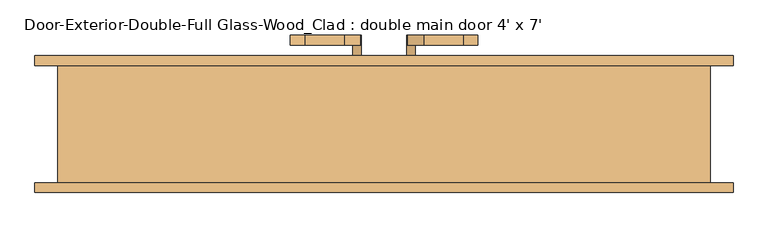
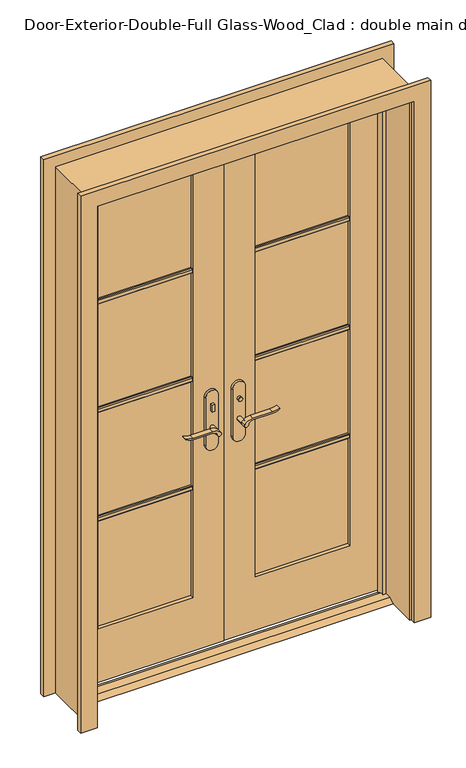
"""IFC4 building model written with IfcOpenShell, lengths in millimetres: door geometry, Door-Exterior-Double-Full Glass-Wood_Clad : double main door 4' x 7'."""

from ifc_helpers import new_model, si_unit, point, frame, frame_2d, origin, place, context, project, spatial, polyline, circle_curve, trimmed, segment, composite_curve, outline, extrude, faceted_brep, source, transform, mapped, element, save


def door_exterior_double_full_glass_wood_clad_double_main_door_4_3788f36b(model_context):
    return source(origin(), model_context, "Body", "SolidModel", [
        extrude(outline(polyline([(19.05, 12.7), (53.975, 12.7), (79.375, 0.0), (-6.35, 0.0), (19.05, 12.7)])), frame((-609.6, 0.0, 0.0), z_axis=(1.0, 0.0, 0.0), x_axis=(0.0, 1.0, 0.0)), (0.0, 0.0, 1.0), 1219.2),
        extrude(outline(polyline([(-47.4019111, 56.2), (-57.4019111, 56.2), (-57.4019111, 66.2), (-47.4019111, 66.2), (-47.4019111, 56.2)])), frame((0.0, 0.0, 981.9), z_axis=(0.0, 0.0, 1.0), x_axis=(1.0, 0.0, 0.0)), (0.0, 0.0, 1.0), 30.0),
        extrude(outline(composite_curve([segment(trimmed(circle_curve(frame_2d((996.9, -52.4019111)), 8.0), [point((996.9, -60.4019111))], [point((996.9, -44.4019111))], False, "CARTESIAN"), True, "CONTINUOUS"), segment(trimmed(circle_curve(frame_2d((996.9, -52.4019111)), 8.0), [point((996.9, -44.4019111))], [point((996.9, -60.4019111))], False, "CARTESIAN"), True, "CONTINUOUS")], self_intersect=False)), frame((0.0, 121.125, 0.0), z_axis=(0.0, 1.0, 0.0), x_axis=(0.0, 0.0, 1.0)), (0.0, 0.0, 1.0), 10.0),
        extrude(outline(composite_curve([segment(trimmed(circle_curve(frame_2d((897.1555521, -76.0694241)), 37.2832219), [point((919.0523287, -45.8937749))], [point((934.4, -77.7693445))], False, "CARTESIAN"), True, "CONTINUOUS"), segment(polyline([(934.4, -77.7693445), (934.4, -154.045502)]), True, "CONTINUOUS"), segment(trimmed(circle_curve(frame_2d((1017.6850638, -153.9791202)), 83.2850902), [point((934.4, -154.045502))], [point((939.4, -182.4019111))], True, "CARTESIAN"), True, "CONTINUOUS"), segment(polyline([(939.4, -182.4019111), (936.6135558, -182.4019111)]), True, "CONTINUOUS"), segment(trimmed(circle_curve(frame_2d((986.6709207, -150.4622499)), 59.3791355), [point((936.6135558, -182.4019111))], [point((927.4, -154.045502))], False, "CARTESIAN"), True, "CONTINUOUS"), segment(polyline([(927.4, -154.045502), (927.4, -77.7881013)]), True, "CONTINUOUS"), segment(trimmed(circle_curve(frame_2d((909.2738613, -77.7881013)), 18.1261387), [point((927.4, -77.7881013))], [point((914.4, -60.4019111))], True, "CARTESIAN"), True, "CONTINUOUS"), segment(trimmed(circle_curve(frame_2d((914.4, -52.4019111)), 8.0), [point((914.4, -60.4019111))], [point((919.0523287, -45.8937749))], False, "CARTESIAN"), True, "CONTINUOUS")], self_intersect=False)), frame((0.0, 16.2, 0.0), z_axis=(0.0, 1.0, 0.0), x_axis=(0.0, 0.0, 1.0)), (0.0, 0.0, 1.0), 20.0),
        extrude(outline(composite_curve([segment(trimmed(circle_curve(frame_2d((914.4, -52.4019111)), 8.0), [point((914.3999903, -60.4019111))], [point((919.0523287, -45.8937749))], False, "CARTESIAN"), True, "CONTINUOUS"), segment(trimmed(circle_curve(frame_2d((897.1555521, -76.0694241)), 37.2832219), [point((919.0523287, -45.8937749))], [point((934.4, -77.7693445))], False, "CARTESIAN"), True, "CONTINUOUS"), segment(polyline([(934.4, -77.7693445), (934.4, -154.045502)]), True, "CONTINUOUS"), segment(trimmed(circle_curve(frame_2d((1017.6850638, -153.9791202)), 83.2850902), [point((934.4, -154.045502))], [point((939.4, -182.4019111))], True, "CARTESIAN"), True, "CONTINUOUS"), segment(polyline([(939.4, -182.4019111), (936.6135558, -182.4019111)]), True, "CONTINUOUS"), segment(trimmed(circle_curve(frame_2d((986.6709207, -150.4622499)), 59.3791355), [point((936.6135558, -182.4019111))], [point((927.4, -154.045502))], False, "CARTESIAN"), True, "CONTINUOUS"), segment(polyline([(927.4, -154.045502), (927.4, -77.788099)]), True, "CONTINUOUS"), segment(trimmed(circle_curve(frame_2d((909.2738682, -77.788099)), 18.1261318), [point((927.4, -77.788099))], [point((914.3999903, -60.4019111))], True, "CARTESIAN"), True, "CONTINUOUS")], self_intersect=False)), frame((0.0, 151.125, 0.0), z_axis=(0.0, 1.0, 0.0), x_axis=(0.0, 0.0, 1.0)), (0.0, 0.0, 1.0), 20.0),
        extrude(outline(composite_curve([segment(trimmed(circle_curve(frame_2d((914.4, -52.4019111)), 8.0), [point((914.4, -60.4019111))], [point((914.4, -44.4019111))], False, "CARTESIAN"), True, "CONTINUOUS"), segment(trimmed(circle_curve(frame_2d((914.4, -52.4019111)), 8.0), [point((914.4, -44.4019111))], [point((914.4, -60.4019111))], False, "CARTESIAN"), True, "CONTINUOUS")], self_intersect=False)), frame((0.0, 36.2, 0.0), z_axis=(0.0, 1.0, 0.0), x_axis=(0.0, 0.0, 1.0)), (0.0, 0.0, 1.0), 30.0),
        extrude(outline(composite_curve([segment(trimmed(circle_curve(frame_2d((914.4, -52.4019111)), 8.0), [point((914.4, -60.4019111))], [point((914.4, -44.4019111))], False, "CARTESIAN"), True, "CONTINUOUS"), segment(trimmed(circle_curve(frame_2d((914.4, -52.4019111)), 8.0), [point((914.4, -44.4019111))], [point((914.4, -60.4019111))], False, "CARTESIAN"), True, "CONTINUOUS")], self_intersect=False)), frame((0.0, 121.125, 0.0), z_axis=(0.0, 1.0, 0.0), x_axis=(0.0, 0.0, 1.0)), (0.0, 0.0, 1.0), 30.0),
        extrude(outline(composite_curve([segment(polyline([(844.4, -27.4019111), (1039.4, -27.4019111)]), True, "CONTINUOUS"), segment(trimmed(circle_curve(frame_2d((1039.4, -52.4019111)), 25.0), [point((1039.4, -27.4019111))], [point((1039.4, -77.4019111))], False, "CARTESIAN"), True, "CONTINUOUS"), segment(polyline([(1039.4, -77.4019111), (844.4, -77.4019111)]), True, "CONTINUOUS"), segment(trimmed(circle_curve(frame_2d((844.4, -52.4019111)), 25.0), [point((844.4, -77.4019111))], [point((844.4, -27.4019111))], False, "CARTESIAN"), True, "CONTINUOUS")], self_intersect=False)), frame((0.0, 66.2, 0.0), z_axis=(0.0, 1.0, 0.0), x_axis=(0.0, 0.0, 1.0)), (0.0, 0.0, 1.0), 10.0),
        extrude(outline(composite_curve([segment(polyline([(844.4, -27.4019111), (1039.4, -27.4019111)]), True, "CONTINUOUS"), segment(trimmed(circle_curve(frame_2d((1039.4, -52.4019111)), 25.0), [point((1039.4, -27.4019111))], [point((1039.4, -77.4019111))], False, "CARTESIAN"), True, "CONTINUOUS"), segment(polyline([(1039.4, -77.4019111), (844.4, -77.4019111)]), True, "CONTINUOUS"), segment(trimmed(circle_curve(frame_2d((844.4, -52.4019111)), 25.0), [point((844.4, -77.4019111))], [point((844.4, -27.4019111))], False, "CARTESIAN"), True, "CONTINUOUS")], self_intersect=False)), frame((0.0, 111.125, 0.0), z_axis=(0.0, 1.0, 0.0), x_axis=(0.0, 0.0, 1.0)), (0.0, 0.0, 1.0), 10.0),
        extrude(outline(polyline([(47.3875, 131.125), (57.3875, 131.125), (57.3875, 121.125), (47.3875, 121.125), (47.3875, 131.125)])), frame((0.0, 0.0, 981.9), z_axis=(0.0, 0.0, 1.0), x_axis=(1.0, 0.0, 0.0)), (0.0, 0.0, 1.0), 30.0),
        extrude(outline(composite_curve([segment(trimmed(circle_curve(frame_2d((996.9, 52.3875)), 8.0), [point((996.9, 60.3875))], [point((996.9, 44.3875))], False, "CARTESIAN"), True, "CONTINUOUS"), segment(trimmed(circle_curve(frame_2d((996.9, 52.3875)), 8.0), [point((996.9, 44.3875))], [point((996.9, 60.3875))], False, "CARTESIAN"), True, "CONTINUOUS")], self_intersect=False)), frame((0.0, 56.2, 0.0), z_axis=(0.0, 1.0, 0.0), x_axis=(0.0, 0.0, 1.0)), (0.0, 0.0, 1.0), 10.0),
        extrude(outline(composite_curve([segment(trimmed(circle_curve(frame_2d((914.4, 52.3875)), 8.0), [point((919.0523287, 45.8793637))], [point((914.4, 60.3875))], False, "CARTESIAN"), True, "CONTINUOUS"), segment(trimmed(circle_curve(frame_2d((909.2738613, 77.7736901)), 18.1261387), [point((914.4, 60.3875))], [point((927.4, 77.7736901))], True, "CARTESIAN"), True, "CONTINUOUS"), segment(polyline([(927.4, 77.7736901), (927.4, 154.0310909)]), True, "CONTINUOUS"), segment(trimmed(circle_curve(frame_2d((986.6709207, 150.4478388)), 59.3791355), [point((927.4, 154.0310909))], [point((936.6135558, 182.3875))], False, "CARTESIAN"), True, "CONTINUOUS"), segment(polyline([(936.6135558, 182.3875), (939.4, 182.3875)]), True, "CONTINUOUS"), segment(trimmed(circle_curve(frame_2d((1017.6850638, 153.9647091)), 83.2850902), [point((939.4, 182.3875))], [point((934.4, 154.0310909))], True, "CARTESIAN"), True, "CONTINUOUS"), segment(polyline([(934.4, 154.0310909), (934.4, 77.7549333)]), True, "CONTINUOUS"), segment(trimmed(circle_curve(frame_2d((897.1555521, 76.0550129)), 37.2832219), [point((934.4, 77.7549333))], [point((919.0523287, 45.8793637))], False, "CARTESIAN"), True, "CONTINUOUS")], self_intersect=False)), frame((0.0, 151.125, 0.0), z_axis=(0.0, 1.0, 0.0), x_axis=(0.0, 0.0, 1.0)), (0.0, 0.0, 1.0), 20.0),
        extrude(outline(composite_curve([segment(trimmed(circle_curve(frame_2d((909.2738682, 77.7736878)), 18.1261318), [point((914.3999903, 60.3875))], [point((927.4, 77.7736878))], True, "CARTESIAN"), True, "CONTINUOUS"), segment(polyline([(927.4, 77.7736878), (927.4, 154.0310909)]), True, "CONTINUOUS"), segment(trimmed(circle_curve(frame_2d((986.6709207, 150.4478388)), 59.3791355), [point((927.4, 154.0310909))], [point((936.6135558, 182.3875))], False, "CARTESIAN"), True, "CONTINUOUS"), segment(polyline([(936.6135558, 182.3875), (939.4, 182.3875)]), True, "CONTINUOUS"), segment(trimmed(circle_curve(frame_2d((1017.6850638, 153.9647091)), 83.2850902), [point((939.4, 182.3875))], [point((934.4, 154.0310909))], True, "CARTESIAN"), True, "CONTINUOUS"), segment(polyline([(934.4, 154.0310909), (934.4, 77.7549333)]), True, "CONTINUOUS"), segment(trimmed(circle_curve(frame_2d((897.1555521, 76.0550129)), 37.2832219), [point((934.4, 77.7549333))], [point((919.0523287, 45.8793637))], False, "CARTESIAN"), True, "CONTINUOUS"), segment(trimmed(circle_curve(frame_2d((914.4, 52.3875)), 8.0), [point((919.0523287, 45.8793637))], [point((914.3999903, 60.3875))], False, "CARTESIAN"), True, "CONTINUOUS")], self_intersect=False)), frame((0.0, 16.2, 0.0), z_axis=(0.0, 1.0, 0.0), x_axis=(0.0, 0.0, 1.0)), (0.0, 0.0, 1.0), 20.0),
        extrude(outline(composite_curve([segment(trimmed(circle_curve(frame_2d((914.4, 52.3875)), 8.0), [point((914.4, 60.3875))], [point((914.4, 44.3875))], False, "CARTESIAN"), True, "CONTINUOUS"), segment(trimmed(circle_curve(frame_2d((914.4, 52.3875)), 8.0), [point((914.4, 44.3875))], [point((914.4, 60.3875))], False, "CARTESIAN"), True, "CONTINUOUS")], self_intersect=False)), frame((0.0, 121.125, 0.0), z_axis=(0.0, 1.0, 0.0), x_axis=(0.0, 0.0, 1.0)), (0.0, 0.0, 1.0), 30.0),
        extrude(outline(composite_curve([segment(trimmed(circle_curve(frame_2d((914.4, 52.3875)), 8.0), [point((914.4, 60.3875))], [point((914.4, 44.3875))], False, "CARTESIAN"), True, "CONTINUOUS"), segment(trimmed(circle_curve(frame_2d((914.4, 52.3875)), 8.0), [point((914.4, 44.3875))], [point((914.4, 60.3875))], False, "CARTESIAN"), True, "CONTINUOUS")], self_intersect=False)), frame((0.0, 36.2, 0.0), z_axis=(0.0, 1.0, 0.0), x_axis=(0.0, 0.0, 1.0)), (0.0, 0.0, 1.0), 30.0),
        extrude(outline(composite_curve([segment(trimmed(circle_curve(frame_2d((844.4, 52.3875)), 25.0), [point((844.4, 27.3875))], [point((844.4, 77.3875))], False, "CARTESIAN"), True, "CONTINUOUS"), segment(polyline([(844.4, 77.3875), (1039.4, 77.3875)]), True, "CONTINUOUS"), segment(trimmed(circle_curve(frame_2d((1039.4, 52.3875)), 25.0), [point((1039.4, 77.3875))], [point((1039.4, 27.3875))], False, "CARTESIAN"), True, "CONTINUOUS"), segment(polyline([(1039.4, 27.3875), (844.4, 27.3875)]), True, "CONTINUOUS")], self_intersect=False)), frame((0.0, 111.125, 0.0), z_axis=(0.0, 1.0, 0.0), x_axis=(0.0, 0.0, 1.0)), (0.0, 0.0, 1.0), 10.0),
        extrude(outline(composite_curve([segment(trimmed(circle_curve(frame_2d((844.4, 52.3875)), 25.0), [point((844.4, 27.3875))], [point((844.4, 77.3875))], False, "CARTESIAN"), True, "CONTINUOUS"), segment(polyline([(844.4, 77.3875), (1039.4, 77.3875)]), True, "CONTINUOUS"), segment(trimmed(circle_curve(frame_2d((1039.4, 52.3875)), 25.0), [point((1039.4, 77.3875))], [point((1039.4, 27.3875))], False, "CARTESIAN"), True, "CONTINUOUS"), segment(polyline([(1039.4, 27.3875), (844.4, 27.3875)]), True, "CONTINUOUS")], self_intersect=False)), frame((0.0, 66.2, 0.0), z_axis=(0.0, 1.0, 0.0), x_axis=(0.0, 0.0, 1.0)), (0.0, 0.0, 1.0), 10.0),
        extrude(outline(polyline([(90.17, 1578.371875), (90.17, 1559.321875), (83.82, 1559.321875), (80.645, 1562.496875), (80.645, 1575.196875), (83.82, 1578.371875), (90.17, 1578.371875)])), frame((120.65, 0.0, 0.0), z_axis=(1.0, 0.0, 0.0), x_axis=(0.0, 1.0, 0.0)), (0.0, 0.0, 1.0), 368.3),
        extrude(outline(polyline([(90.17, 1132.68125), (90.17, 1113.63125), (83.82, 1113.63125), (80.645, 1116.80625), (80.645, 1129.50625), (83.82, 1132.68125), (90.17, 1132.68125)])), frame((120.65, 0.0, 0.0), z_axis=(1.0, 0.0, 0.0), x_axis=(0.0, 1.0, 0.0)), (0.0, 0.0, 1.0), 368.3),
        extrude(outline(polyline([(90.17, 686.990625), (90.17, 667.940625), (83.82, 667.940625), (80.645, 671.115625), (80.645, 683.815625), (83.82, 686.990625), (90.17, 686.990625)])), frame((120.65, 0.0, 0.0), z_axis=(1.0, 0.0, 0.0), x_axis=(0.0, 1.0, 0.0)), (0.0, 0.0, 1.0), 368.3),
        extrude(outline(polyline([(97.155, 1578.371875), (103.505, 1578.371875), (106.68, 1575.196875), (106.68, 1562.496875), (103.505, 1559.321875), (97.155, 1559.321875), (97.155, 1578.371875)])), frame((-488.95, 0.0, 0.0), z_axis=(1.0, 0.0, 0.0), x_axis=(0.0, 1.0, 0.0)), (0.0, 0.0, 1.0), 368.3),
        extrude(outline(polyline([(97.155, 1132.68125), (103.505, 1132.68125), (106.68, 1129.50625), (106.68, 1116.80625), (103.505, 1113.63125), (97.155, 1113.63125), (97.155, 1132.68125)])), frame((-488.95, 0.0, 0.0), z_axis=(1.0, 0.0, 0.0), x_axis=(0.0, 1.0, 0.0)), (0.0, 0.0, 1.0), 368.3),
        extrude(outline(polyline([(97.155, 686.990625), (103.505, 686.990625), (106.68, 683.815625), (106.68, 671.115625), (103.505, 667.940625), (97.155, 667.940625), (97.155, 686.990625)])), frame((-488.95, 0.0, 0.0), z_axis=(1.0, 0.0, 0.0), x_axis=(0.0, 1.0, 0.0)), (0.0, 0.0, 1.0), 368.3),
        extrude(outline(polyline([(97.155, 1578.371875), (103.505, 1578.371875), (106.68, 1575.196875), (106.68, 1562.496875), (103.505, 1559.321875), (97.155, 1559.321875), (97.155, 1578.371875)])), frame((120.65, 0.0, 0.0), z_axis=(1.0, 0.0, 0.0), x_axis=(0.0, 1.0, 0.0)), (0.0, 0.0, 1.0), 368.3),
        extrude(outline(polyline([(97.155, 1132.68125), (103.505, 1132.68125), (106.68, 1129.50625), (106.68, 1116.80625), (103.505, 1113.63125), (97.155, 1113.63125), (97.155, 1132.68125)])), frame((120.65, 0.0, 0.0), z_axis=(1.0, 0.0, 0.0), x_axis=(0.0, 1.0, 0.0)), (0.0, 0.0, 1.0), 368.3),
        extrude(outline(polyline([(97.155, 686.990625), (103.505, 686.990625), (106.68, 683.815625), (106.68, 671.115625), (103.505, 667.940625), (97.155, 667.940625), (97.155, 686.990625)])), frame((120.65, 0.0, 0.0), z_axis=(1.0, 0.0, 0.0), x_axis=(0.0, 1.0, 0.0)), (0.0, 0.0, 1.0), 368.3),
        extrude(outline(polyline([(90.17, 1578.371875), (90.17, 1559.321875), (83.82, 1559.321875), (80.645, 1562.496875), (80.645, 1575.196875), (83.82, 1578.371875), (90.17, 1578.371875)])), frame((-488.95, 0.0, 0.0), z_axis=(1.0, 0.0, 0.0), x_axis=(0.0, 1.0, 0.0)), (0.0, 0.0, 1.0), 368.3),
        extrude(outline(polyline([(90.17, 1132.68125), (90.17, 1113.63125), (83.82, 1113.63125), (80.645, 1116.80625), (80.645, 1129.50625), (83.82, 1132.68125), (90.17, 1132.68125)])), frame((-488.95, 0.0, 0.0), z_axis=(1.0, 0.0, 0.0), x_axis=(0.0, 1.0, 0.0)), (0.0, 0.0, 1.0), 368.3),
        extrude(outline(polyline([(90.17, 686.990625), (90.17, 667.940625), (83.82, 667.940625), (80.645, 671.115625), (80.645, 683.815625), (83.82, 686.990625), (90.17, 686.990625)])), frame((-488.95, 0.0, 0.0), z_axis=(1.0, 0.0, 0.0), x_axis=(0.0, 1.0, 0.0)), (0.0, 0.0, 1.0), 368.3),
        extrude(outline(polyline([(0.0, 615.95), (0.0, 679.45), (2203.45, 679.45), (2203.45, -679.45), (0.0, -679.45), (0.0, -615.95), (2139.95, -615.95), (2139.95, 615.95), (0.0, 615.95)])), frame((0.0, -136.525, 0.0), z_axis=(0.0, 1.0, 0.0), x_axis=(0.0, 0.0, 1.0)), (0.0, 0.0, 1.0), 19.05),
        extrude(outline(polyline([(0.0, 615.95), (0.0, 679.45), (2203.45, 679.45), (2203.45, -679.45), (0.0, -679.45), (0.0, -615.95), (2139.95, -615.95), (2139.95, 615.95), (0.0, 615.95)])), frame((0.0, 111.125, 0.0), z_axis=(0.0, 1.0, 0.0), x_axis=(0.0, 0.0, 1.0)), (0.0, 0.0, 1.0), 19.05),
        faceted_brep([(635.0, 111.125, 0.0), (635.0, -117.475, 0.0), (609.6, -117.475, 0.0), (609.6, 41.275, 0.0), (596.9, 41.275, 0.0), (596.9, 76.2, 0.0), (609.6, 76.2, 0.0), (609.6, 111.125, 0.0), (635.0, 111.125, 2159.0), (635.0, -117.475, 2159.0), (-635.0, -117.475, 2159.0), (-635.0, -117.475, 0.0), (-609.6, -117.475, 0.0), (-609.6, -117.475, 2133.6), (609.6, -117.475, 2133.6), (609.6, 41.275, 2133.6), (-609.6, 41.275, 2133.6), (-609.6, 41.275, 0.0), (-596.9, 41.275, 0.0), (-596.9, 41.275, 2120.9), (596.9, 41.275, 2120.9), (596.9, 76.2, 2120.9), (1.5875, 76.2, 2120.9), (-1.6019111, 76.2, 2120.9), (-596.9, 76.2, 2120.9), (-596.9, 76.2, 0.0), (-609.6, 76.2, 0.0), (-609.6, 76.2, 2133.6), (-1.6019111, 76.2, 2133.6), (1.5875, 76.2, 2133.6), (609.6, 76.2, 2133.6), (609.6, 111.125, 2133.6), (1.5875, 111.125, 2133.6), (-1.6019111, 111.125, 2133.6), (-609.6, 111.125, 2133.6), (-609.6, 111.125, 0.0), (-635.0, 111.125, 0.0), (-635.0, 111.125, 2159.0)], [[[0, 1, 2, 3, 4, 5, 6, 7]], [[1, 0, 8, 9]], [[2, 1, 9, 10, 11, 12, 13, 14]], [[3, 2, 14, 15]], [[4, 3, 15, 16, 17, 18, 19, 20]], [[5, 4, 20, 21]], [[6, 5, 21, 22, 23, 24, 25, 26, 27, 28, 29, 30]], [[7, 6, 30, 31]], [[0, 7, 31, 32, 33, 34, 35, 36, 37, 8]], [[9, 8, 37, 10]], [[14, 13, 16, 15]], [[20, 19, 24, 23, 22, 21]], [[31, 30, 29, 28, 27, 34, 33, 32]], [[12, 11, 36, 35, 26, 25, 18, 17]], [[11, 10, 37, 36]], [[13, 12, 17, 16]], [[19, 18, 25, 24]], [[27, 26, 35, 34]]]),
        extrude(outline(polyline([(12.7, 609.6), (2133.6, 609.6), (2133.6, 1.5875), (12.7, 1.5875), (12.7, 609.6)]), holes=[polyline([(2014.5375, 120.65), (2014.5375, 488.95), (231.775, 488.95), (231.775, 120.65), (2014.5375, 120.65)])]), frame((0.0, 76.2, 0.0), z_axis=(0.0, 1.0, 0.0), x_axis=(0.0, 0.0, 1.0)), (0.0, 0.0, 1.0), 34.925),
        extrude(outline(polyline([(2133.6, -609.6), (12.7, -609.6), (12.7, -1.6019111), (2133.6, -1.6019111), (2133.6, -609.6)]), holes=[polyline([(231.775, -488.95), (2014.5375, -488.95), (2014.5375, -120.65), (231.775, -120.65), (231.775, -488.95)])]), frame((0.0, 76.2, 0.0), z_axis=(0.0, 1.0, 0.0), x_axis=(0.0, 0.0, 1.0)), (0.0, 0.0, 1.0), 34.925),
        extrude(outline(polyline([(488.95, 90.17), (120.65, 90.17), (120.65, 97.155), (488.95, 97.155), (488.95, 90.17)])), frame((0.0, 0.0, 231.775), z_axis=(0.0, 0.0, 1.0), x_axis=(1.0, 0.0, 0.0)), (0.0, 0.0, 1.0), 1782.7625),
        extrude(outline(polyline([(-120.65, 90.17), (-488.95, 90.17), (-488.95, 97.155), (-120.65, 97.155), (-120.65, 90.17)])), frame((0.0, 0.0, 231.775), z_axis=(0.0, 0.0, 1.0), x_axis=(1.0, 0.0, 0.0)), (0.0, 0.0, 1.0), 1782.7625),
    ])


if __name__ == "__main__":
    model = new_model("IFC4")
    model_context = context("Model", 3, world=origin())
    ifc_project = project(units=[si_unit("LENGTHUNIT", "METRE", prefix="MILLI")], contexts=[model_context])
    site = spatial("IfcSite", under=ifc_project)
    building = spatial("IfcBuilding", under=site)
    placement = place(None, origin())
    door_exterior_double_full_glass_wood_clad_double_main_door_4_shape = door_exterior_double_full_glass_wood_clad_double_main_door_4_3788f36b(model_context)
    element("IfcDoor", 1, ObjectType="Door-Exterior-Double-Full Glass-Wood_Clad : double main door 4' x 7'", at=placement, inside=building, context=model_context, shape_type="MappedRepresentation", body=[
        mapped(door_exterior_double_full_glass_wood_clad_double_main_door_4_shape, transform((0.0, 0.0, 0.0), x_axis=(1.0, 0.0, 0.0), y_axis=(0.0, 1.0, 0.0), z_axis=(0.0, 0.0, 1.0))),
    ])
    save(model, "model.ifc")

# Revit data of these elements
# Type "Door-Exterior-Double-Full Glass-Wood_Clad : double main door 4' x 7'"
#   Type Mark = "14"
#   Assembly Code = "B2030100"
#   Analytic Construction = "French door, wood frame with double glass"
#   Top Rail = 0' - 4 11/16"
#   Threshold Offset [instance default] = 0' - 0 1/2"
#   Thickness = 0' - 1 3/8"
#   Thermal Resistance (R) = 1.9158 (h·ft²·°F)/BTU
#   Swing Angle [instance default] = 90.00°
#   Stiles = 0' - 4 3/4"
#   Rough Width = 4' - 2"
#   Rough Height = 7' - 1"
#   Panel Width = 2' - 0"
#   Door Offset [instance default] = 0' - 0"
#   Height = 7' - 0"
#   Width = 4' - 0"
#   Heat Transfer Coefficient (U) = 0.5220 BTU/(h·ft²·°F)
#   Bottom Rail = 0' - 9 1/8"
#   Exterior Trim [instance default] = yes
#   Threshold [instance default] = yes
#   Show Grill [instance default] = yes
#   Function = 1
#   Trim Material = Cherry
#   Threshold Material = Cherry
#   Panel Material = Cherry
#   Glazing = Glass
#   Frame Material = Cherry
#   Door Handle Material = Aluminum
#   Visual Light Transmittance = 0
#   Solar Heat Gain Coefficient = 0
#   Wall Closure = (empty or 0)
#   Construction Type = (empty or 0)
# Element 1 (IfcDoor, "Door-Exterior-Double-Full Glass-Wood_Clad : double main door 4' x 7'")
#   Materials on its faces: "Cherry", "Aluminum", "Glass"
# Materials
#   "Cherry": class "Wood", colour RGB 226 177 128, transparency 0, Description = "Prunus Serotina", Cost = 0
#   "Glass": class "Glass", colour RGB 0 128 192, transparency 0.75, Description = "Soda Lime Glass", Cost = 0
#   "Aluminum": class "Metal", colour RGB 247 247 247, transparency 0, Description = "Aluminum 6061", Cost = 0
